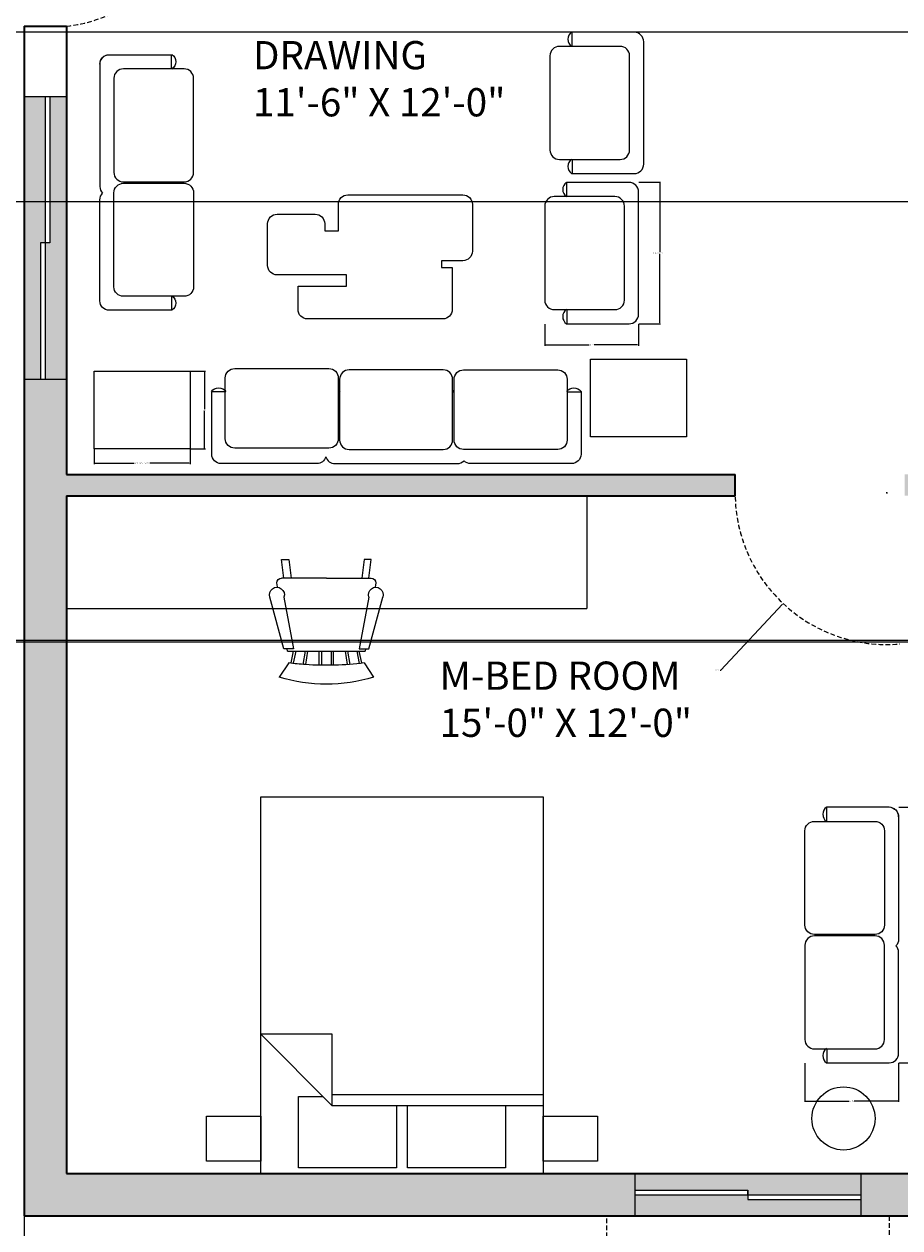
# Model space of a CAD drawing. Units: inches. Extents: x 1693 to 2974, y 2201 to 2965.
# Tile 17 of 24: x 2479 to 2665, y 2332 to 2588. Entities that reach past the tile are written whole.
import ezdxf

# ---------------------------------------------------------------- set-up
doc = ezdxf.new("R2010")
doc.units = ezdxf.units.IN
doc.header["$LTSCALE"] = 2
doc.header["$MEASUREMENT"] = 0
doc.linetypes.add('HIDDEN', pattern=[0.375, 0.25, -0.125])
for name, color, linetype, lineweight in [('A-ANNO-DIMS', 2, 'Continuous', 18), ('A-AREA-IDEN', 7, 'Continuous', 18), ('A-DOOR-SWNG', 3, 'HIDDEN', 13), ('A-FLOR-CASE', 32, 'Continuous', 18), ('A-FURN', 8, 'Continuous', 18), ('A-GLAZ', 4, 'Continuous', 18), ('A-GLAZ-OVHD', 8, 'HIDDEN', 13), ('A-WALL', 7, 'Continuous', 35)]:
    doc.layers.add(name, color=color, linetype=linetype, lineweight=lineweight)
doc.layers.add('A-GLAZ-PATT', color=141, linetype='Continuous', lineweight=13, true_color=0xadddf7)
doc.layers.add('A-WALL-PATT', color=251, linetype='Continuous', lineweight=13, true_color=0x636466)
doc.styles.get("Standard").update_dxf_attribs({"font": 'arial.ttf'})
doc.dimstyles.get("Standard").update_dxf_attribs({"dimtxt": 0.18, "dimasz": 0.18, "dimexe": 0.18, "dimexo": 0.0625, "dimgap": 0.09, "dimtad": 0, "dimtih": 1, "dimtoh": 1, "dimdec": 1, "dimzin": 0, "dimdsep": 46, "dimlunit": 3, "dimtxsty": 'Standard', "dimcen": 0.09, "dimadec": 0, "dimazin": 0, "dimtfac": 1, "dimtdec": 1, "dimtofl": 0, "dimtmove": 0, "dimatfit": 3, "dimfxl": 1, "dimtolj": 1, "dimtzin": 0, "dimarcsym": 0})

# ---------------------------------------------------------------- blocks, each defined once
blk = doc.blocks.new('Chair - Rocking')
for p, q in [((-8, -4.5), (-10, -1.5)), ((8, -4.5), (10, -1.5)), ((-7.5, -4.5), (-7, -7)), ((-6.5, -7), (-7.02225, -4.43)), ((-4.5, -7), (-4.96674, -4.19951)), ((-4, -7), (-4.40532, -4.16272)), ((-1.5, -4.05012), (-1.5, -7)), ((-1, -7), (-1, -4.05012)), ((1, -7), (1, -4.04655)), ((1.5, -4.05012), (1.5, -7)), ((4, -7), (4.40187, -4.18694)), ((4.5, -7), (4.96761, -4.19437)), ((6.5, -7), (7, -4.4057)), ((7.5, -4.5), (7, -7)), ((-9, -7.5), (-12, -18.49999)), ((-7, -7.5), (-9, -7.5)), ((-9, -18.49999), (-7, -7.5)), ((-8.23428, -6.99939), (-8.3093, -7.47958)), ((-8.23041, -7), (8.23915, -7)), ((7, -7.5), (9, -7.5)), ((9, -18.49999), (7, -7.5)), ((8.31071, -7.48854), (8.23449, -7.00073)), ((9, -7.5), (12, -18.49999)), ((-10.36644, -20.64523), (-10.5, -21.49999)), ((-9, -22.49999), (-9.5, -26.49999)), ((0, -22.49999), (-9.5, -22.49999)), ((-8, -26.49999), (-7.5, -22.49999)), ((0, -22.49999), (9.5, -22.49999)), ((8, -26.49999), (7.5, -22.49999)), ((9, -22.49999), (9.5, -26.49999)), ((10.5, -21.49999), (10.3575, -20.58798)), ((-9.5, -26.49999), (-8, -26.49999)), ((9.5, -26.49999), (8, -26.49999))]:
    blk.add_line(p, q)
for centre, radius, start, end in [((0, -34.08333), 34.08333, 72.93847, 107.0615), ((0, -68.25004), 64.25, 93.92211, 97.15267), ((0, -68.25004), 64.25, 82.84733, 93.92211), ((-10.5, -18.99999), 1.58114, 161.5651, 18.43495), ((10.5, -18.99999), 1.58114, 161.5651, 18.43495), ((-9.5, -21.49999), 1, 180, 270), ((9.5, -21.49999), 1, 270, 0)]:
    blk.add_arc(centre, radius, start, end)
blk = doc.blocks.new('Bed - Queen')
for p, q in [((0, -80.00003), (0, 0)), ((0, 0), (59.99999, 0)), ((59.99999, 0), (59.99999, -80.00003)), ((7.99999, -1.2), (28.79998, -1.2)), ((7.99999, -14.4), (7.99999, -1.2)), ((28.79998, -1.2), (28.79998, -14.4)), ((31.19999, -1.2), (51.99999, -1.2)), ((31.19999, -14.4), (31.19999, -1.2)), ((51.99999, -1.2), (51.99999, -16.4)), ((0, -14.4), (44.8, -14.4)), ((59.99999, -29.6), (44.8, -14.4)), ((44.8, -14.4), (44.8, -29.6)), ((44.8, -16.8), (0, -16.8)), ((51.99999, -16.4), (46.79936, -16.4)), ((44.8, -29.6), (59.99999, -29.6)), ((59.99999, -80.00003), (0, -80.00003))]:
    blk.add_line(p, q)
blk = doc.blocks.new('SOFA-2-SEAT')
at = {"ltscale": 2}
for p, q in [((17.9, 54.27), (4.68, 54.27)), ((4.68, 51.27), (4.68, 54.27)), ((4.68, 51.27), (4.68, 51.55)), ((4.68, 27.26), (4.68, 26.96)), ((19.9, 2), (19.9, 23.43)), ((4.68, 3), (4.68, 0)), ((4.59, 0), (17.9, 0))]:
    blk.add_line(p, q, dxfattribs=at)
for points in [[(18.47, 54.18, -0.331344), (19.9, 52.27), (19.9, 26.26, -0.198912), (19.31, 24.85)], [(0, 49.27, -0.414214), (2, 51.27), (14.9, 51.27, -0.414214), (16.9, 49.27), (16.9, 29.26, -0.414214), (14.9, 27.26), (2, 27.26, -0.414214), (0, 29.26), (0, 49.27)], [(0, 4.95, 0.414214), (2, 2.95), (14.9, 2.95, 0.414214), (16.9, 4.95), (16.9, 24.96, 0.414214), (14.9, 26.96), (2, 26.96, 0.414214), (0, 24.96), (0, 4.95)]]:
    blk.add_lwpolyline(points, format="xyb", dxfattribs=at)
for centre, radius, start, end in [((5.65, 52.79), 1.86, 125.0084, 234.9916), ((17.9, 52.27), 2, 0, 90), ((5.65, 52.75), 1.86, 219.881, 234.9916), ((5.65, 25.74), 1.86, 125.0084, 139.1343), ((17.9, 23.43), 2, 0, 45), ((5.65, 1.52), 1.86, 125.0084, 234.9916), ((17.9, 2), 2, 270, 0)]:
    blk.add_arc(centre, radius, start, end, dxfattribs=at)
blk = doc.blocks.new('SOFA-3-SEAT')
at = {"ltscale": 2}
for p, q in [((0.05, 18.19), (0.05, 4.98)), ((22.37, 20.19), (2.05, 20.19)), ((76.47, 20.19), (55.04, 20.19)), ((78.47, 4.88), (78.47, 18.19)), ((3.05, 4.98), (0.05, 4.98)), ((27.21, 4.98), (26.92, 4.98)), ((51.21, 4.98), (51.52, 4.98)), ((75.47, 4.98), (78.47, 4.98))]:
    blk.add_line(p, q, dxfattribs=at)
for points in [[(24.29, 18.76, -0.331344), (26.21, 20.19), (52.21, 20.19, -0.198912), (53.63, 19.6)], [(24.92, 0, 0.414214), (26.92, 2), (26.92, 14.9, 0.414214), (24.92, 16.9), (4.92, 16.9, 0.414214), (2.92, 14.9), (2.92, 2, 0.414214), (4.92, 0), (24.92, 0)], [(29.21, 0.29, -0.414214), (27.21, 2.29), (27.21, 15.19, -0.414214), (29.21, 17.19), (49.21, 17.19, -0.414214), (51.21, 15.19), (51.21, 2.29, -0.414214), (49.21, 0.29), (29.21, 0.29)], [(73.52, 0.29, 0.414214), (75.52, 2.29), (75.52, 15.19, 0.414214), (73.52, 17.19), (53.52, 17.19, 0.414214), (51.52, 15.19), (51.52, 2.29, 0.414214), (53.52, 0.29), (73.52, 0.29)]]:
    blk.add_lwpolyline(points, format="xyb", dxfattribs=at)
for centre, radius, start, end in [((2.05, 18.19), 2, 90, 180), ((22.37, 18.19), 2, 16.6709, 90), ((55.04, 18.19), 2, 90, 135), ((76.47, 18.19), 2, 0, 90), ((1.52, 5.95), 1.86, 215.0084, 324.9916), ((25.73, 5.95), 1.86, 309.881, 324.9916), ((52.73, 5.95), 1.86, 215.0084, 229.1343), ((76.95, 5.95), 1.86, 215.0084, 324.9916)]:
    blk.add_arc(centre, radius, start, end, dxfattribs=at)
blk = doc.blocks.new('LOUNGE-CHAIR-B')
at = {"ltscale": 2}
for p, q in [((4.68, 27.01), (4.68, 30.01)), ((4.68, 3), (4.68, 0))]:
    blk.add_line(p, q, dxfattribs=at)
for points in [[(4.59, 0), (17.9, 0, 0.414214), (19.9, 2), (19.9, 28.01, 0.414214), (17.9, 30.01), (4.68, 30.01)], [(0, 5, 0.414214), (2, 3), (14.9, 3, 0.414214), (16.9, 5), (16.9, 25.01, 0.414214), (14.9, 27.01), (2, 27.01, 0.414214), (0, 25.01), (0, 5)]]:
    blk.add_lwpolyline(points, format="xyb", dxfattribs=at)
for centre in [(5.66, 28.53), (5.66, 1.52)]:
    blk.add_arc(centre, 1.86, 125.0084, 234.9916, dxfattribs=at)
blk = doc.blocks.new('NIGHTSTAND')
at = {"ltscale": 2}
blk.add_lwpolyline([(11.51, 0), (0, 0), (0, 9.62), (11.51, 9.62)], close=True, dxfattribs=at)
blk = doc.blocks.new('TABLE-COCKTAIL')
at = {"ltscale": 2}
blk.add_lwpolyline([(17.32, 26.34), (41.47, 26.34, -0.414214), (43.47, 24.34), (43.47, 14.36, -0.414214), (41.47, 12.36), (36.89, 12.36), (36.89, 10.89), (39.2, 10.89), (39.2, 2, -0.414214), (37.2, 0), (8.45, 0, -0.414214), (6.45, 2), (6.45, 6.97), (16.72, 6.97), (16.72, 9.34), (2, 9.34, -0.414214), (0, 11.34), (0, 20.23, -0.414214), (2, 22.23), (10.11, 22.23, -0.414214), (12.11, 20.23), (12.11, 18.68), (15.01, 18.68), (15.01, 24.34, -0.414214), (17.01, 26.34), (17.32, 26.34)], format="xyb", dxfattribs=at)
blk = doc.blocks.new('TABLE-END-RECT')
at = {"ltscale": 2}
blk.add_lwpolyline([(0, 16.48), (20.41, 16.48), (20.41, 0), (0, 0)], close=True, dxfattribs=at)
blk = doc.blocks.new('TABLE-END-ROUND')
at = {"ltscale": 2}
blk.add_circle((6.71, 6.71), 6.71, dxfattribs=at)
blk = doc.blocks.new('*D47')
at = {"layer": 'A-ANNO-DIMS', "color": 0, "lineweight": -2, "ltscale": 2, "transparency": 16777216}
for p, q in [((2665.02, 2421.61), (2673.28, 2421.61)), ((2673.1, 2421.43), (2673.1, 2394.63)), ((2673.1, 2367.47), (2673.1, 2394.27)), ((2665.02, 2367.29), (2673.28, 2367.29))]:
    blk.add_line(p, q, dxfattribs=at)
at = {"layer": 'A-ANNO-DIMS', "color": 0, "ltscale": 2, "transparency": 16777216}
for points in [[(2673.07, 2421.43), (2673.13, 2421.43), (2673.1, 2421.61)], [(2673.07, 2367.47), (2673.13, 2367.47), (2673.1, 2367.29)]]:
    blk.add_solid(points, dxfattribs=at)
at = {"layer": 'Defpoints', "color": 0, "ltscale": 2, "transparency": 16777216}
for p in [(2664.96, 2421.61), (2673.1, 2421.61), (2664.96, 2367.29)]:
    blk.add_point(p, dxfattribs=at)
at = {"layer": 'A-ANNO-DIMS', "color": 0, "ltscale": 2, "transparency": 16777216, "insert": (2673.1, 2394.45), "char_height": 0.18, "attachment_point": 5}
blk.add_mtext('\\A1;TWO-SEAT SOFA 54 TYP.', dxfattribs=at)
blk = doc.blocks.new('*D48')
at = {"layer": 'A-ANNO-DIMS', "color": 0, "lineweight": -2, "ltscale": 2, "transparency": 16777216}
for p, q in [((2645.06, 2367.23), (2645.06, 2358.97)), ((2664.96, 2367.23), (2664.96, 2358.97)), ((2645.24, 2359.15), (2654.48, 2359.15)), ((2664.78, 2359.15), (2655.54, 2359.15))]:
    blk.add_line(p, q, dxfattribs=at)
at = {"layer": 'A-ANNO-DIMS', "color": 0, "ltscale": 2, "transparency": 16777216}
for points in [[(2645.24, 2359.18), (2645.24, 2359.12), (2645.06, 2359.15)], [(2664.78, 2359.18), (2664.78, 2359.12), (2664.96, 2359.15)]]:
    blk.add_solid(points, dxfattribs=at)
at = {"layer": 'Defpoints', "color": 0, "ltscale": 2, "transparency": 16777216}
for p in [(2645.06, 2367.29), (2664.96, 2367.29), (2664.96, 2359.15)]:
    blk.add_point(p, dxfattribs=at)
at = {"layer": 'A-ANNO-DIMS', "color": 0, "ltscale": 2, "transparency": 16777216, "insert": (2655.01, 2359.15), "char_height": 0.18, "attachment_point": 5}
blk.add_mtext('\\A1;20 TYP.', dxfattribs=at)
blk = doc.blocks.new('*D67')
at = {"layer": 'A-ANNO-DIMS', "color": 0, "lineweight": -2, "ltscale": 2, "transparency": 16777216}
for p, q in [((2609.78, 2554.32), (2614.41, 2554.32)), ((2614.23, 2554.14), (2614.23, 2539.48)), ((2614.23, 2524.45), (2614.23, 2539.11)), ((2609.78, 2524.27), (2614.41, 2524.27))]:
    blk.add_line(p, q, dxfattribs=at)
at = {"layer": 'A-ANNO-DIMS', "color": 0, "ltscale": 2, "transparency": 16777216}
for points in [[(2614.2, 2554.14), (2614.26, 2554.14), (2614.23, 2554.32)], [(2614.2, 2524.45), (2614.26, 2524.45), (2614.23, 2524.27)]]:
    blk.add_solid(points, dxfattribs=at)
at = {"layer": 'Defpoints', "color": 0, "ltscale": 2, "transparency": 16777216}
for p in [(2609.72, 2554.32), (2614.23, 2554.32), (2609.72, 2524.27)]:
    blk.add_point(p, dxfattribs=at)
at = {"layer": 'A-ANNO-DIMS', "color": 0, "ltscale": 2, "transparency": 16777216, "insert": (2614.23, 2539.3), "char_height": 0.18, "attachment_point": 5}
blk.add_mtext('\\A1;LOUNGE CHAIR B 30 TYP.', dxfattribs=at)
blk = doc.blocks.new('*D68')
at = {"layer": 'A-ANNO-DIMS', "color": 0, "lineweight": -2, "ltscale": 2, "transparency": 16777216}
for p, q in [((2589.82, 2524.21), (2589.82, 2519.58)), ((2609.72, 2524.21), (2609.72, 2519.58)), ((2590, 2519.76), (2599.24, 2519.76)), ((2609.54, 2519.76), (2600.3, 2519.76))]:
    blk.add_line(p, q, dxfattribs=at)
at = {"layer": 'A-ANNO-DIMS', "color": 0, "ltscale": 2, "transparency": 16777216}
for points in [[(2590, 2519.79), (2590, 2519.73), (2589.82, 2519.76)], [(2609.54, 2519.79), (2609.54, 2519.73), (2609.72, 2519.76)]]:
    blk.add_solid(points, dxfattribs=at)
at = {"layer": 'Defpoints', "color": 0, "ltscale": 2, "transparency": 16777216}
for p in [(2589.82, 2524.27), (2609.72, 2524.27), (2609.72, 2519.76)]:
    blk.add_point(p, dxfattribs=at)
at = {"layer": 'A-ANNO-DIMS', "color": 0, "ltscale": 2, "transparency": 16777216, "insert": (2599.77, 2519.76), "char_height": 0.18, "attachment_point": 5}
blk.add_mtext('\\A1;20 TYP.', dxfattribs=at)
blk = doc.blocks.new('*D73')
at = {"layer": 'A-ANNO-DIMS', "color": 0, "lineweight": -2, "ltscale": 2, "transparency": 16777216}
for p, q in [((2494.1, 2497.64), (2494.1, 2494.46)), ((2514.51, 2497.64), (2514.51, 2494.46)), ((2494.28, 2494.64), (2502.64, 2494.64)), ((2514.33, 2494.64), (2505.97, 2494.64))]:
    blk.add_line(p, q, dxfattribs=at)
at = {"layer": 'A-ANNO-DIMS', "color": 0, "ltscale": 2, "transparency": 16777216}
for points in [[(2494.28, 2494.67), (2494.28, 2494.61), (2494.1, 2494.64)], [(2514.33, 2494.67), (2514.33, 2494.61), (2514.51, 2494.64)]]:
    blk.add_solid(points, dxfattribs=at)
at = {"layer": 'Defpoints', "color": 0, "ltscale": 2, "transparency": 16777216}
for p in [(2494.1, 2497.7), (2514.51, 2497.7), (2514.51, 2494.64)]:
    blk.add_point(p, dxfattribs=at)
at = {"layer": 'A-ANNO-DIMS', "color": 0, "ltscale": 2, "transparency": 16777216, "insert": (2504.31, 2494.64), "char_height": 0.18, "attachment_point": 5}
blk.add_mtext('\\A1;RECT. END TABLE 20 TYP.', dxfattribs=at)
blk = doc.blocks.new('*D74')
at = {"layer": 'A-ANNO-DIMS', "color": 0, "lineweight": -2, "ltscale": 2, "transparency": 16777216}
for p, q in [((2514.57, 2514.18), (2517.75, 2514.18)), ((2517.57, 2514), (2517.57, 2506.12)), ((2517.57, 2497.88), (2517.57, 2505.76)), ((2514.57, 2497.7), (2517.75, 2497.7))]:
    blk.add_line(p, q, dxfattribs=at)
at = {"layer": 'A-ANNO-DIMS', "color": 0, "ltscale": 2, "transparency": 16777216}
for points in [[(2517.54, 2514), (2517.6, 2514), (2517.57, 2514.18)], [(2517.54, 2497.88), (2517.6, 2497.88), (2517.57, 2497.7)]]:
    blk.add_solid(points, dxfattribs=at)
at = {"layer": 'Defpoints', "color": 0, "ltscale": 2, "transparency": 16777216}
for p in [(2514.51, 2514.18), (2517.57, 2514.18), (2514.51, 2497.7)]:
    blk.add_point(p, dxfattribs=at)
at = {"layer": 'A-ANNO-DIMS', "color": 0, "ltscale": 2, "transparency": 16777216, "insert": (2517.57, 2505.94), "char_height": 0.18, "attachment_point": 5}
blk.add_mtext('\\A1;16 TYP.', dxfattribs=at)
blk = doc.blocks.new('*D81')
at = {"layer": 'A-ANNO-DIMS', "color": 0, "lineweight": -2, "ltscale": 2, "transparency": 16777216}
for p, q in [((1752.34, 2553.91), (1752.34, 2964.96)), ((1752.52, 2964.78), (2332.94, 2964.78)), ((2914.06, 2964.78), (2333.64, 2964.78)), ((2914.24, 2754.97), (2914.24, 2964.96))]:
    blk.add_line(p, q, dxfattribs=at)
at = {"layer": 'A-ANNO-DIMS', "color": 0, "ltscale": 2, "transparency": 16777216}
for points in [[(1752.52, 2964.81), (1752.52, 2964.75), (1752.34, 2964.78)], [(2914.06, 2964.81), (2914.06, 2964.75), (2914.24, 2964.78)]]:
    blk.add_solid(points, dxfattribs=at)
at = {"layer": 'Defpoints', "color": 0, "ltscale": 2, "transparency": 16777216}
for p in [(2914.24, 2964.78), (2914.24, 2754.9), (1752.34, 2553.84)]:
    blk.add_point(p, dxfattribs=at)
at = {"layer": 'A-ANNO-DIMS', "color": 0, "ltscale": 2, "transparency": 16777216, "insert": (2333.29, 2964.78), "char_height": 0.18, "attachment_point": 5}
blk.add_mtext('\\A1;1162', dxfattribs=at)
blk = doc.blocks.new('*D82')
at = {"layer": 'A-ANNO-DIMS', "color": 0, "lineweight": -2, "ltscale": 2, "transparency": 16777216}
for p, q in [((2615.67, 2906.08), (1693.46, 2906.08)), ((1693.64, 2905.9), (1693.64, 2582.94)), ((1693.64, 2259.62), (1693.64, 2582.58)), ((2096.17, 2259.44), (1693.46, 2259.44))]:
    blk.add_line(p, q, dxfattribs=at)
at = {"layer": 'A-ANNO-DIMS', "color": 0, "ltscale": 2, "transparency": 16777216}
for points in [[(1693.61, 2905.9), (1693.67, 2905.9), (1693.64, 2906.08)], [(1693.61, 2259.62), (1693.67, 2259.62), (1693.64, 2259.44)]]:
    blk.add_solid(points, dxfattribs=at)
at = {"layer": 'Defpoints', "color": 0, "ltscale": 2, "transparency": 16777216}
for p in [(1693.64, 2906.08), (2615.74, 2906.08), (2096.24, 2259.44)]:
    blk.add_point(p, dxfattribs=at)
at = {"layer": 'A-ANNO-DIMS', "color": 0, "ltscale": 2, "transparency": 16777216, "insert": (1693.64, 2582.76), "char_height": 0.18, "attachment_point": 5}
blk.add_mtext('\\A1;646.6', dxfattribs=at)
blk = doc.blocks.new('*D85')
at = {"layer": 'A-ANNO-DIMS', "color": 0, "lineweight": -2, "ltscale": 2, "transparency": 16777216}
for p, q in [((2479.24, 2334.69), (2479.24, 2200.56)), ((2902.24, 2334.69), (2902.24, 2200.56)), ((2479.42, 2200.74), (2690.44, 2200.74)), ((2902.06, 2200.74), (2691.03, 2200.74))]:
    blk.add_line(p, q, dxfattribs=at)
at = {"layer": 'A-ANNO-DIMS', "color": 0, "ltscale": 2, "transparency": 16777216}
for points in [[(2479.42, 2200.77), (2479.42, 2200.71), (2479.24, 2200.74)], [(2902.06, 2200.77), (2902.06, 2200.71), (2902.24, 2200.74)]]:
    blk.add_solid(points, dxfattribs=at)
at = {"layer": 'Defpoints', "color": 0, "ltscale": 2, "transparency": 16777216}
for p in [(2479.24, 2334.75), (2902.24, 2334.75), (2902.24, 2200.74)]:
    blk.add_point(p, dxfattribs=at)
at = {"layer": 'A-ANNO-DIMS', "color": 0, "ltscale": 2, "transparency": 16777216, "insert": (2690.74, 2200.74), "char_height": 0.18, "attachment_point": 5}
blk.add_mtext('\\A1;423', dxfattribs=at)
blk = doc.blocks.new('*D89')
at = {"layer": 'A-ANNO-DIMS', "color": 0, "lineweight": -2, "ltscale": 2, "transparency": 16777216}
for p, q in [((2479.3, 2334.75), (2973.12, 2334.75)), ((2972.94, 2334.57), (2972.94, 2312.48)), ((2972.94, 2290.02), (2972.94, 2312.12)), ((2294.3, 2289.84), (2973.12, 2289.84))]:
    blk.add_line(p, q, dxfattribs=at)
at = {"layer": 'A-ANNO-DIMS', "color": 0, "ltscale": 2, "transparency": 16777216}
for points in [[(2972.91, 2334.57), (2972.97, 2334.57), (2972.94, 2334.75)], [(2972.91, 2290.02), (2972.97, 2290.02), (2972.94, 2289.84)]]:
    blk.add_solid(points, dxfattribs=at)
at = {"layer": 'Defpoints', "color": 0, "ltscale": 2, "transparency": 16777216}
for p in [(2479.24, 2334.75), (2972.94, 2334.75), (2294.24, 2289.84)]:
    blk.add_point(p, dxfattribs=at)
at = {"layer": 'A-ANNO-DIMS', "color": 0, "ltscale": 2, "transparency": 16777216, "insert": (2972.94, 2312.3), "char_height": 0.18, "attachment_point": 5}
blk.add_mtext('\\A1;44.91', dxfattribs=at)
blk = doc.blocks.new('*D96')
at = {"layer": 'A-ANNO-DIMS', "color": 0, "lineweight": -2, "ltscale": 2, "transparency": 16777216}
for p, q in [((2294.3, 2586.26), (2973.12, 2586.26)), ((2972.94, 2586.08), (2972.94, 2568.45)), ((2972.94, 2550.44), (2972.94, 2568.08)), ((2294.3, 2550.26), (2973.12, 2550.26))]:
    blk.add_line(p, q, dxfattribs=at)
at = {"layer": 'A-ANNO-DIMS', "color": 0, "ltscale": 2, "transparency": 16777216}
for points in [[(2972.91, 2586.08), (2972.97, 2586.08), (2972.94, 2586.26)], [(2972.91, 2550.44), (2972.97, 2550.44), (2972.94, 2550.26)]]:
    blk.add_solid(points, dxfattribs=at)
at = {"layer": 'Defpoints', "color": 0, "ltscale": 2, "transparency": 16777216}
for p in [(2294.24, 2586.26), (2972.94, 2586.26), (2294.24, 2550.26)]:
    blk.add_point(p, dxfattribs=at)
at = {"layer": 'A-ANNO-DIMS', "color": 0, "ltscale": 2, "transparency": 16777216, "insert": (2972.94, 2568.26), "char_height": 0.18, "attachment_point": 5}
blk.add_mtext('\\A1;36', dxfattribs=at)
blk = doc.blocks.new('*D97')
at = {"layer": 'A-ANNO-DIMS', "color": 0, "lineweight": -2, "ltscale": 2, "transparency": 16777216}
for p, q in [((2294.3, 2631.75), (2973.12, 2631.75)), ((2972.94, 2631.57), (2972.94, 2609.19)), ((2972.94, 2586.44), (2972.94, 2608.83)), ((2294.3, 2586.26), (2973.12, 2586.26))]:
    blk.add_line(p, q, dxfattribs=at)
at = {"layer": 'A-ANNO-DIMS', "color": 0, "ltscale": 2, "transparency": 16777216}
for points in [[(2972.91, 2631.57), (2972.97, 2631.57), (2972.94, 2631.75)], [(2972.91, 2586.44), (2972.97, 2586.44), (2972.94, 2586.26)]]:
    blk.add_solid(points, dxfattribs=at)
at = {"layer": 'Defpoints', "color": 0, "ltscale": 2, "transparency": 16777216}
for p in [(2294.24, 2631.75), (2972.94, 2631.75), (2294.24, 2586.26)]:
    blk.add_point(p, dxfattribs=at)
at = {"layer": 'A-ANNO-DIMS', "color": 0, "ltscale": 2, "transparency": 16777216, "insert": (2972.94, 2609.01), "char_height": 0.18, "attachment_point": 5}
blk.add_mtext('\\A1;45.49', dxfattribs=at)
blk = doc.blocks.new('*D108')
at = {"layer": 'A-ANNO-DIMS', "color": 0, "lineweight": -2, "ltscale": 2, "transparency": 16777216}
for p, q in [((2972.94, 2457.27), (2972.94, 2457.45)), ((2972.94, 2457.45), (2973.12, 2457.45)), ((1752.74, 2457.09), (2973.12, 2457.09)), ((1752.74, 2456.73), (2973.12, 2456.73)), ((2972.94, 2456.55), (2972.94, 2456.37))]:
    blk.add_line(p, q, dxfattribs=at)
at = {"layer": 'A-ANNO-DIMS', "color": 0, "ltscale": 2, "transparency": 16777216}
for points in [[(2972.91, 2457.27), (2972.97, 2457.27), (2972.94, 2457.09)], [(2972.91, 2456.55), (2972.97, 2456.55), (2972.94, 2456.73)]]:
    blk.add_solid(points, dxfattribs=at)
at = {"layer": 'Defpoints', "color": 0, "ltscale": 2, "transparency": 16777216}
for p in [(1752.68, 2457.09), (1752.68, 2456.73), (2972.94, 2457.09)]:
    blk.add_point(p, dxfattribs=at)
at = {"layer": 'A-ANNO-DIMS', "color": 0, "ltscale": 2, "transparency": 16777216, "insert": (2973.44, 2457.45), "char_height": 0.18, "attachment_point": 5}
blk.add_mtext('\\A1;0.36', dxfattribs=at)
blk = doc.blocks.new('*D115')
at = {"layer": 'A-ANNO-DIMS', "color": 0, "lineweight": -2, "ltscale": 2, "transparency": 16777216}
for p, q in [((2662.4, 2488.39), (2662.58, 2488.39)), ((2662.49, 2488.3), (2662.49, 2488.48)), ((2627.21, 2450.72), (2640.31, 2464.72)), ((2627.03, 2450.72), (2627.21, 2450.72))]:
    blk.add_line(p, q, dxfattribs=at)
at = {"layer": 'A-ANNO-DIMS', "color": 0, "ltscale": 2, "transparency": 16777216}
blk.add_solid([(2640.29, 2464.74), (2640.34, 2464.7), (2640.44, 2464.85)], dxfattribs=at)
at = {"layer": 'Defpoints', "color": 0, "ltscale": 2, "transparency": 16777216}
for p in [(2662.49, 2488.39), (2640.44, 2464.85)]:
    blk.add_point(p, dxfattribs=at)
at = {"layer": 'A-ANNO-DIMS', "color": 0, "ltscale": 2, "transparency": 16777216, "insert": (2626.48, 2450.72), "char_height": 0.18, "attachment_point": 5}
blk.add_mtext('\\A1;R32.256', dxfattribs=at)

msp = doc.modelspace()

# ---------------------------------------------------------------- hatches: boundary and pattern name
at = {"layer": 'A-GLAZ-PATT', "ltscale": 2}
h = msp.add_hatch(color=256, dxfattribs=at)
h.dxf.hatch_style = 1
h.paths.add_polyline_path([(2656.9702, 2338.2547), (2632.9702, 2338.2547), (2632.9702, 2339.2547), (2608.9702, 2339.2547), (2608.9702, 2334.7547), (2656.9702, 2334.7547)])
h.paths.add_polyline_path([(2656.9702, 2343.7547), (2608.9702, 2343.7547), (2608.9702, 2340.2547), (2632.9702, 2340.2547), (2632.9702, 2339.2547), (2656.9702, 2339.2547)])
h.paths.add_polyline_path([(2775.7544, 2338.2547), (2751.7544, 2338.2547), (2751.7544, 2334.7547), (2775.7544, 2334.7547)])
h.paths.add_polyline_path([(2775.7544, 2343.7547), (2751.7544, 2343.7547), (2751.7544, 2340.2547), (2775.7544, 2340.2547)])
h.paths.add_polyline_path([(2897.7363, 2568.7999), (2893.2363, 2568.7999), (2893.2363, 2520.7999), (2896.7363, 2520.7999), (2896.7363, 2544.7999), (2897.7363, 2544.7999)])
h.paths.add_polyline_path([(2902.2363, 2568.7999), (2898.7363, 2568.7999), (2898.7363, 2544.7999), (2897.7363, 2544.7999), (2897.7363, 2520.7999), (2902.2363, 2520.7999)])
h.paths.add_polyline_path([(2902.2363, 2637.7547), (2898.7363, 2637.7547), (2898.7363, 2613.7547), (2902.2363, 2613.7547)])
h.paths.add_polyline_path([(2896.7363, 2637.7547), (2893.2363, 2637.7547), (2893.2363, 2613.7547), (2896.7363, 2613.7547)])
h.paths.add_polyline_path([(2902.2363, 2748.903), (2899.0477, 2748.903), (2899.0477, 2724.903), (2898.0477, 2724.903), (2898.0477, 2700.903), (2902.2363, 2700.903)])
h.paths.add_polyline_path([(2898.0477, 2748.903), (2893.2363, 2748.903), (2893.2363, 2700.903), (2897.0477, 2700.903), (2897.0477, 2724.903), (2898.0477, 2724.903)])
h.paths.add_polyline_path([(2851.2363, 2846.2547), (2803.2363, 2846.2547), (2803.2363, 2842.7547), (2827.2363, 2842.7547), (2827.2363, 2841.7547), (2851.2363, 2841.7547)])
h.paths.add_polyline_path([(2851.2363, 2840.7547), (2827.2363, 2840.7547), (2827.2363, 2841.7547), (2803.2363, 2841.7547), (2803.2363, 2837.2547), (2851.2363, 2837.2547)])
h.paths.add_polyline_path([(2578.2363, 2846.2547), (2530.2363, 2846.2547), (2530.2363, 2842.7547), (2554.2363, 2842.7547), (2554.2363, 2841.7547), (2578.2363, 2841.7547)])
h.paths.add_polyline_path([(2578.2363, 2840.7547), (2554.2363, 2840.7547), (2554.2363, 2841.7547), (2530.2363, 2841.7547), (2530.2363, 2837.2547), (2578.2363, 2837.2547)])
h.paths.add_polyline_path([(2732.7363, 2812.7547), (2705.1363, 2812.7547), (2705.1363, 2811.7547), (2676.3363, 2811.7547), (2676.3363, 2812.7547), (2648.7363, 2812.7547), (2648.7363, 2808.2547), (2732.7363, 2808.2547)])
h.paths.add_polyline_path([(2732.7363, 2817.2547), (2648.7363, 2817.2547), (2648.7363, 2813.7547), (2676.3363, 2813.7547), (2676.3363, 2812.7547), (2705.1363, 2812.7547), (2705.1363, 2813.7547), (2732.7363, 2813.7547)])
h.paths.add_polyline_path([(2488.2363, 2695.8203), (2484.7878, 2695.8203), (2484.7878, 2671.8203), (2488.2363, 2671.8203)])
h.paths.add_polyline_path([(2482.7878, 2695.8203), (2479.2363, 2695.8203), (2479.2363, 2671.8203), (2482.7878, 2671.8203)])
h.paths.add_polyline_path([(2488.2363, 2572.4371), (2484.7363, 2572.4371), (2484.7363, 2541.4371), (2483.7363, 2541.4371), (2483.7363, 2512.4371), (2488.2363, 2512.4371)])
h.paths.add_polyline_path([(2482.7363, 2541.4371), (2483.7363, 2541.4371), (2483.7363, 2572.4371), (2479.2363, 2572.4371), (2479.2363, 2512.4371), (2482.7363, 2512.4371)])
h.paths.add_polyline_path([(2248.9863, 2706.8449), (2190.9863, 2706.8449), (2190.9863, 2703.3449), (2219.9863, 2703.3449), (2219.9863, 2702.3449), (2248.9863, 2702.3449)])
h.paths.add_polyline_path([(2248.9863, 2701.3449), (2219.9863, 2701.3449), (2219.9863, 2702.3449), (2190.9863, 2702.3449), (2190.9863, 2697.8449), (2248.9863, 2697.8449)])
h.paths.add_polyline_path([(2151.9207, 2293.3449), (2127.9207, 2293.3449), (2127.9207, 2289.8449), (2151.9207, 2289.8449)])
h.paths.add_polyline_path([(2151.9207, 2298.8449), (2127.9207, 2298.8449), (2127.9207, 2295.3449), (2151.9207, 2295.3449)])
h.paths.add_polyline_path([(2084.023, 2293.3449), (2066.023, 2293.3449), (2066.023, 2294.3449), (2048.023, 2294.3449), (2048.023, 2289.8449), (2084.023, 2289.8449)])
h.paths.add_polyline_path([(2084.023, 2298.8449), (2048.023, 2298.8449), (2048.023, 2295.3449), (2066.023, 2295.3449), (2066.023, 2294.3449), (2084.023, 2294.3449)])
h.paths.add_polyline_path([(1966.0781, 2293.3449), (1948.0781, 2293.3449), (1948.0781, 2294.3449), (1930.0781, 2294.3449), (1930.0781, 2289.8449), (1966.0781, 2289.8449)])
h.paths.add_polyline_path([(1966.0781, 2298.8449), (1930.0781, 2298.8449), (1930.0781, 2295.3449), (1948.0781, 2295.3449), (1948.0781, 2294.3449), (1966.0781, 2294.3449)])
h.paths.add_polyline_path([(1787.2363, 2403.1922), (1782.7363, 2403.1922), (1782.7363, 2355.1922), (1786.2363, 2355.1922), (1786.2363, 2379.1922), (1787.2363, 2379.1922)])
h.paths.add_polyline_path([(1791.7363, 2403.1922), (1788.2363, 2403.1922), (1788.2363, 2379.1922), (1787.2363, 2379.1922), (1787.2363, 2355.1922), (1791.7363, 2355.1922)])
h.paths.add_polyline_path([(1786.2363, 2477.5455), (1782.7363, 2477.5455), (1782.7363, 2453.5455), (1786.2363, 2453.5455)])
h.paths.add_polyline_path([(1791.7363, 2477.5455), (1788.2363, 2477.5455), (1788.2363, 2453.5455), (1791.7363, 2453.5455)])
h.paths.add_polyline_path([(1786.2363, 2621.6433), (1782.7363, 2621.6433), (1782.7363, 2585.6433), (1786.2363, 2585.6433)])
h.paths.add_polyline_path([(1791.7363, 2621.6433), (1788.2363, 2621.6433), (1788.2363, 2585.6433), (1791.7363, 2585.6433)])
h.paths.add_polyline_path([(1908.1286, 2706.8449), (1860.1286, 2706.8449), (1860.1286, 2703.3449), (1884.1286, 2703.3449), (1884.1286, 2702.3449), (1908.1286, 2702.3449)])
h.paths.add_polyline_path([(1908.1286, 2701.3449), (1884.1286, 2701.3449), (1884.1286, 2702.3449), (1860.1286, 2702.3449), (1860.1286, 2697.8449), (1908.1286, 2697.8449)])
h.paths.add_polyline_path([(1973.9863, 2706.8449), (1949.9863, 2706.8449), (1949.9863, 2703.3449), (1973.9863, 2703.3449)])
h.paths.add_polyline_path([(1973.9863, 2701.3449), (1949.9863, 2701.3449), (1949.9863, 2697.8449), (1973.9863, 2697.8449)])
h.paths.add_polyline_path([(2112.7363, 2690.3449), (2028.7363, 2690.3449), (2028.7363, 2686.8449), (2056.3363, 2686.8449), (2056.3363, 2685.8449), (2085.1363, 2685.8449), (2085.1363, 2686.8449), (2112.7363, 2686.8449)])
h.paths.add_polyline_path([(2112.7363, 2685.8449), (2085.1363, 2685.8449), (2085.1363, 2684.8449), (2056.3363, 2684.8449), (2056.3363, 2685.8449), (2028.7363, 2685.8449), (2028.7363, 2681.3449), (2112.7363, 2681.3449)])
h.paths.add_polyline_path([(2422.7363, 2640.7547), (2350.7363, 2640.7547), (2350.7363, 2637.2547), (2386.7363, 2637.2547), (2386.7363, 2636.2547), (2422.7363, 2636.2547)])
h.paths.add_polyline_path([(2422.7363, 2635.2547), (2386.7363, 2635.2547), (2386.7363, 2636.2547), (2350.7363, 2636.2547), (2350.7363, 2631.7547), (2422.7363, 2631.7547)])
at = {"layer": 'A-WALL-PATT', "ltscale": 2}
h = msp.add_hatch(color=256, dxfattribs=at)
h.dxf.hatch_style = 1
h.paths.add_polyline_path([(1928.2363, 2733.2161), (1930.9384, 2733.2161), (1930.9384, 2737.2161), (1923.7363, 2737.2161), (1923.7363, 2706.8449), (1908.1286, 2706.8449), (1908.1286, 2697.8449), (1923.7363, 2697.8449), (1923.7363, 2692.8449), (1928.2363, 2692.8449), (1928.2363, 2697.8449), (1949.9863, 2697.8449), (1949.9863, 2706.8449), (1928.2363, 2706.8449)])
h.paths.add_polyline_path([(2004.7363, 2737.2161), (1995.7363, 2737.2161), (1995.7363, 2706.8449), (1985.6374, 2706.8449), (1973.9863, 2706.8449), (1973.9863, 2697.8449), (2000.2363, 2697.8449), (2000.2363, 2686.5348), (2000.3613, 2686.5348), (2000.3613, 2667.0432), (2000.2363, 2601.8449), (1928.2363, 2601.8449), (1928.2363, 2662.8449), (1923.7363, 2662.8449), (1923.7363, 2595.3449), (1928.2363, 2595.3449), (1928.2363, 2597.3449), (2004.7363, 2597.3449), (2004.7363, 2681.3449), (2012.7814, 2681.3449), (2028.7363, 2681.3449), (2028.7363, 2690.3449), (2004.7363, 2690.3449)])
h.paths.add_polyline_path([(2190.9863, 2706.8449), (2184.9863, 2706.8449), (2145.7363, 2706.8449), (2145.7363, 2765.3449), (2145.7363, 2774.5394), (2136.7363, 2774.5394), (2136.7363, 2756.3449), (2136.7363, 2690.3449), (2112.7363, 2690.3449), (2112.7363, 2681.3449), (2136.7363, 2681.3449), (2136.7363, 2597.3449), (2141.2363, 2597.3449), (2141.2363, 2697.8449), (2190.9863, 2697.8449)])
h.paths.add_polyline_path([(1860.1286, 2706.8449), (1782.7363, 2706.8449), (1782.7363, 2621.6433), (1791.7363, 2621.6433), (1791.7363, 2697.8449), (1860.1286, 2697.8449)])
h.paths.add_polyline_path([(1791.7363, 2585.6433), (1782.7363, 2585.6433), (1782.7363, 2562.8449), (1782.7363, 2553.8449), (1752.3363, 2553.8449), (1752.3363, 2544.2586), (1756.3363, 2544.2586), (1756.3363, 2549.3449), (1782.7363, 2549.3449), (1782.7363, 2489.2404), (1782.7363, 2477.5455), (1791.7363, 2477.5455), (1791.7363, 2493.5991), (1791.6113, 2493.5991), (1791.6113, 2513.0907), (1791.6824, 2533.7198, -0.94742783), (1791.7363, 2534.7168), (1791.7363, 2549.3449), (1863.7363, 2549.3449), (1863.7363, 2513.3449), (1866.7363, 2513.3449), (1866.7363, 2549.3449), (1924.7363, 2549.3449), (1924.7363, 2447.3449), (1924.7363, 2442.8449), (1933.7363, 2442.8449), (1933.7363, 2447.3449), (1928.2363, 2447.3449), (1928.2363, 2559.3449), (1923.7363, 2559.3449), (1923.7363, 2553.8449), (1791.7363, 2553.8449), (1791.7363, 2562.8449)])
h.paths.add_polyline_path([(1791.7363, 2442.8449), (1866.7363, 2442.8449), (1866.7363, 2447.3449), (1866.7363, 2483.3449), (1863.7363, 2483.3449), (1863.7363, 2447.3449), (1791.7363, 2447.3449), (1791.7363, 2453.5455), (1782.7363, 2453.5455), (1782.7363, 2447.3449), (1756.3363, 2447.3449), (1756.3363, 2455.7126), (1752.3363, 2455.7126), (1752.3363, 2442.8449), (1782.7363, 2442.8449), (1782.7363, 2403.1922), (1791.7363, 2403.1922)])
h.paths.add_polyline_path([(1930.0781, 2298.8449), (1791.7363, 2298.8449), (1791.7363, 2355.1922), (1782.7363, 2355.1922), (1782.7363, 2289.8449), (1930.0781, 2289.8449)])
h.paths.add_polyline_path([(2624.7363, 2883.2547), (2624.7363, 2902.6165), (2624.7363, 2906.0761), (2615.7363, 2906.0761), (2615.7363, 2892.2547), (2615.7363, 2846.2547), (2578.2363, 2846.2547), (2578.2363, 2837.2547), (2620.2363, 2837.2547), (2620.2363, 2743.2547), (2624.7363, 2743.2547), (2624.7363, 2808.2547), (2648.7363, 2808.2547), (2648.7363, 2817.2547), (2624.7363, 2817.2547)])
h.paths.add_polyline_path([(2530.2363, 2846.2547), (2479.2363, 2846.2547), (2479.2363, 2695.8203), (2488.2363, 2695.8203), (2488.2363, 2700.7547), (2567.2363, 2700.7547), (2567.2363, 2705.2547), (2488.2363, 2705.2547), (2488.2363, 2837.2547), (2530.2363, 2837.2547)])
h.paths.add_polyline_path([(2488.2363, 2487.7547), (2630.2363, 2487.7547, -0.00990191), (2630.2363, 2489.0322), (2630.2363, 2492.2547), (2488.2363, 2492.2547), (2488.2363, 2512.4371), (2479.2363, 2512.4371), (2479.2363, 2334.7547), (2608.9702, 2334.7547), (2608.9702, 2343.7547), (2488.2363, 2343.7547)])
h.paths.add_polyline_path([(2751.7544, 2343.7547), (2672.7363, 2343.7547), (2672.7363, 2409.7547), (2674.7363, 2409.7547), (2674.7363, 2413.7547), (2672.7363, 2413.7547), (2672.7363, 2487.7547), (2732.7363, 2487.7547), (2732.7363, 2413.7547), (2704.7363, 2413.7547), (2704.7363, 2409.7547), (2784.7363, 2409.7547), (2784.7363, 2343.7547), (2775.7544, 2343.7547), (2775.7544, 2334.7547), (2902.2363, 2334.7547), (2902.2363, 2520.7999), (2893.2363, 2520.7999), (2893.2363, 2413.7547), (2856.0145, 2413.7547), (2856.0145, 2409.7547), (2893.2363, 2409.7547), (2893.2363, 2343.7547), (2789.2363, 2343.7547), (2789.2363, 2409.7547), (2819.2363, 2409.7547), (2826.0145, 2409.7547), (2826.0145, 2413.7547), (2789.2363, 2413.7547), (2789.2363, 2492.2547), (2784.7363, 2492.2547), (2784.7363, 2413.7547), (2736.7363, 2413.7547), (2736.7363, 2492.2547), (2672.7363, 2492.2547), (2666.2363, 2492.2547), (2666.2363, 2487.7547), (2668.2363, 2487.7547), (2668.2363, 2343.7547), (2656.9702, 2343.7547), (2656.9702, 2334.7547), (2662.9702, 2334.7547), (2751.7544, 2334.7547)])
h.paths.add_polyline_path([(2902.2363, 2613.7547), (2893.2363, 2613.7547), (2893.2363, 2589.7547), (2785.2363, 2589.7547), (2785.2363, 2661.7547), (2790.2363, 2661.7547), (2790.2363, 2665.2547), (2761.2363, 2665.2547), (2761.2363, 2667.2547), (2756.7363, 2667.2547), (2756.7363, 2661.7547), (2781.2363, 2661.7547), (2781.2363, 2585.7547), (2893.2363, 2585.7547), (2893.2363, 2568.7999), (2902.2363, 2568.7999)])
h.paths.add_polyline_path([(2488.2363, 2671.8203), (2479.2363, 2671.8203), (2479.2363, 2645.2547), (2479.2363, 2623.4598), (2488.2363, 2623.4598), (2488.2363, 2636.2547), (2624.7363, 2636.2547), (2624.7363, 2640.7547), (2603.7363, 2640.7547), (2603.7363, 2700.7547), (2624.7363, 2700.7547), (2624.7363, 2707.2547), (2620.2363, 2707.2547), (2620.2363, 2705.2547), (2597.2363, 2705.2547), (2597.2363, 2700.7547), (2599.2363, 2700.7547), (2599.2363, 2640.7547), (2488.2363, 2640.7547)])
h.paths.add_polyline_path([(2761.2363, 2837.2547), (2803.2363, 2837.2547), (2803.2363, 2846.2547), (2797.2363, 2846.2547), (2765.7363, 2846.2547), (2756.7363, 2846.2547), (2756.7363, 2817.2547), (2732.7363, 2817.2547), (2732.7363, 2808.2547), (2756.7363, 2808.2547), (2756.7363, 2703.2547), (2761.2363, 2703.2547)])
h.paths.add_polyline_path([(2739.7489, 2433.1234), (2786.9181, 2433.1234), (2786.9181, 2455.5122), (2739.7489, 2455.5122)], flags=25)

# ---------------------------------------------------------------- linework, layer by layer
at = {"layer": 'A-DOOR-SWNG', "ltscale": 2}
for centre, radius, start, end in [((2484.8526, 2618.1226), 30.8489, 276.297258, 9.962947), ((2662.4862, 2488.3934), 32.2562, 178.865361, 274.890936)]:
    msp.add_arc(centre, radius, start, end, dxfattribs=at)
at = {"layer": 'A-FLOR-CASE', "ltscale": 2}
for p in [(2598.7493, 2487.7547), (2488.2363, 2463.7547)]:
    msp.add_line(p, (2598.7493, 2463.7547), dxfattribs=at)
at = {"layer": 'A-GLAZ', "ltscale": 2}
for p, q in [((2488.2363, 2572.4371), (2479.2363, 2572.4371)), ((2483.7363, 2572.4371), (2483.7363, 2512.4371)), ((2484.7363, 2572.4371), (2484.7363, 2541.4371)), ((2484.7363, 2541.4371), (2482.7363, 2541.4371)), ((2482.7363, 2541.4371), (2482.7363, 2512.4371)), ((2488.2363, 2512.4371), (2479.2363, 2512.4371)), ((2608.9702, 2343.7547), (2608.9702, 2334.7547)), ((2656.9702, 2343.7547), (2656.9702, 2334.7547)), ((2608.9702, 2340.2547), (2632.9702, 2340.2547)), ((2632.9702, 2339.2547), (2632.9702, 2340.2547)), ((2632.9702, 2340.2547), (2632.9702, 2338.2547)), ((2608.9702, 2339.2547), (2656.9702, 2339.2547)), ((2632.9702, 2338.2547), (2656.9702, 2338.2547))]:
    msp.add_line(p, q, dxfattribs=at)
at = {"layer": 'A-GLAZ-OVHD', "ltscale": 2}
for p, q in [((2602.9702, 2322.7547), (2602.9702, 2334.7547)), ((2656.9702, 2334.7547), (2662.9702, 2334.7547)), ((2662.9702, 2334.7547), (2662.9702, 2322.7547))]:
    msp.add_line(p, q, dxfattribs=at)
at = {"layer": 'A-WALL', "ltscale": 2}
for p, q in [((2479.2363, 2587.4598), (2488.2363, 2587.4598)), ((2488.2363, 2492.2547), (2630.2363, 2492.2547)), ((2630.2363, 2487.7547), (2630.2363, 2492.2547)), ((2488.2363, 2487.7547), (2630.2363, 2487.7547)), ((2488.2363, 2343.7547), (2668.2363, 2343.7547)), ((2479.2363, 2334.7547), (2902.2363, 2334.7547))]:
    msp.add_line(p, q, dxfattribs=at)
at = {"layer": 'A-WALL'}
for p, q in [((2479.2363, 2587.4598), (2479.2363, 2334.7547)), ((2488.2363, 2587.4598), (2488.2363, 2492.2547)), ((2488.2363, 2487.7547), (2488.2363, 2343.7547))]:
    msp.add_line(p, q, dxfattribs=at)

# ---------------------------------------------------------------- block references
at = {"layer": 'A-FURN'}
for name, p in [('LOUNGE-CHAIR-B', (2590.922, 2556.172)), ('LOUNGE-CHAIR-B', (2589.8232, 2524.27)), ('TABLE-COCKTAIL', (2530.9641, 2525.3099)), ('TABLE-END-RECT', (2599.5163, 2500.2608)), ('TABLE-END-RECT', (2494.1, 2497.702)), ('SOFA-2-SEAT', (2645.0611, 2367.2945)), ('TABLE-END-ROUND', (2646.5377, 2348.7646)), ('NIGHTSTAND', (2517.986, 2346.3688)), ('NIGHTSTAND', (2589.4958, 2346.3688))]:
    msp.add_blockref(name, p, dxfattribs=at)
at = {"layer": 'A-FURN', "extrusion": (0, 0, -1), "zscale": -1}
msp.add_blockref('SOFA-2-SEAT', (-2515.2214, 2527.1478), dxfattribs=at)
at = {"layer": 'A-FURN', "extrusion": (0, 0, -1), "zscale": -1, "rotation": 180}
msp.add_blockref('SOFA-3-SEAT', (-2519.0415, 2514.7595), dxfattribs=at)
at = {"layer": 'A-FURN', "ltscale": 2, "xscale": -1, "rotation": 180}
msp.add_blockref('Chair - Rocking', (2543.4303, 2447.7205), dxfattribs=at)
at = {"layer": 'A-FURN', "ltscale": 2, "rotation": 180}
msp.add_blockref('Bed - Queen', (2589.4959, 2343.7547), dxfattribs=at)

# ---------------------------------------------------------------- texts
at = {"layer": 'A-AREA-IDEN', "ltscale": 2, "char_height": 6, "attachment_point": 1}
for s, insert in [('DRAWING\\P11\'-6" X 12\'-0"', (2527.8505, 2584.3187)), ('M-BED ROOM\\P15\'-0" X 12\'-0"', (2567.4805, 2452.519))]:
    msp.add_mtext_dynamic_manual_height_columns(s, width=108.452746, gutter_width=1, heights=[0], dxfattribs=dict(at, insert=insert))

# ---------------------------------------------------------------- dimensions: what is measured, and where the dimension line sits
at = {"layer": 'A-ANNO-DIMS', "ltscale": 2}
for base, p1, p2, picture, middle in [((2914.2363, 2964.7761), (1752.3363, 2553.8449), (2914.2363, 2754.903), '*D81', (2333.2863, 2964.7761)), ((2902.2363, 2200.7449), (2479.2363, 2334.7547), (2902.2363, 2334.7547), '*D85', (2690.7363, 2200.7449))]:
    dim = msp.add_linear_dim(base=base, p1=p1, p2=p2, dimstyle='Standard', override={"dimdec": 0, "dimlfac": 1, "dimrnd": 0, "dimzin": 0, "dimdsep": 46, "dimlunit": 2}, dxfattribs=at)
    dim.commit()
    dim.dimension.update_dxf_attribs({"geometry": picture, "text_midpoint": middle})
for base, p1, p2, override, picture, middle in [((1693.6363, 2906.0761), (2096.2363, 2259.4449), (2615.7363, 2906.0761), {"dimdec": 1, "dimlfac": 1, "dimrnd": 0, "dimzin": 0, "dimdsep": 46, "dimlunit": 2}, '*D82', (1693.6363, 2582.7605)), ((2972.9363, 2631.7547), (2294.2363, 2586.2648), (2294.2363, 2631.7547), {"dimdec": 2, "dimlfac": 1, "dimrnd": 0, "dimzin": 0, "dimdsep": 46, "dimlunit": 2}, '*D97', (2972.9363, 2609.0097)), ((2972.9363, 2586.2648), (2294.2363, 2550.2648), (2294.2363, 2586.2648), {"dimdec": 0, "dimlfac": 1, "dimrnd": 0, "dimzin": 0, "dimdsep": 46, "dimlunit": 2}, '*D96', (2972.9363, 2568.2648)), ((2972.9363, 2457.0877), (1752.6754, 2456.7302), (1752.6754, 2457.0877), {"dimdec": 2, "dimlfac": 1, "dimrnd": 0, "dimzin": 0, "dimdsep": 46, "dimlunit": 2}, '*D108', (2973.44, 2457.4477)), ((2972.9363, 2334.7547), (2294.2363, 2289.8449), (2479.2363, 2334.7547), {"dimdec": 2, "dimlfac": 1, "dimrnd": 0, "dimzin": 0, "dimdsep": 46, "dimlunit": 2}, '*D89', (2972.9363, 2312.2998))]:
    dim = msp.add_linear_dim(base=base, p1=p1, p2=p2, angle=90, dimstyle='Standard', override=override, dxfattribs=at)
    dim.commit()
    dim.dimension.update_dxf_attribs({"geometry": picture, "text_midpoint": middle})
for base, p1, p2, text, picture, middle in [((2614.2263, 2554.32), (2609.7188, 2524.2701), (2609.7188, 2554.32), 'LOUNGE CHAIR B <> TYP.', '*D67', (2614.2263, 2539.2951)), ((2517.5726, 2514.1818), (2514.511, 2497.7022), (2514.511, 2514.1818), '<> TYP.', '*D74', (2517.5726, 2505.942)), ((2673.1032, 2421.6075), (2664.9563, 2367.2948), (2664.9563, 2421.6075), 'TWO-SEAT SOFA <> TYP.', '*D47', (2673.1032, 2394.4511))]:
    dim = msp.add_linear_dim(base=base, p1=p1, p2=p2, angle=90, text=text, dimstyle='Standard', override={"dimdec": 0, "dimlfac": 1, "dimrnd": 0, "dimzin": 0, "dimdsep": 46, "dimlunit": 2}, dxfattribs=at)
    dim.commit()
    dim.dimension.update_dxf_attribs({"geometry": picture, "text_midpoint": middle})
for base, p1, p2, text, picture, middle in [((2609.7188, 2519.7627), (2589.8235, 2524.2701), (2609.7188, 2524.2701), '<> TYP.', '*D68', (2599.7712, 2519.7627)), ((2514.511, 2494.6406), (2494.1002, 2497.7022), (2514.511, 2497.7022), 'RECT. END TABLE <> TYP.', '*D73', (2504.3056, 2494.6406)), ((2664.9563, 2359.1479), (2645.061, 2367.2948), (2664.9563, 2367.2948), '<> TYP.', '*D48', (2655.0086, 2359.1479))]:
    dim = msp.add_linear_dim(base=base, p1=p1, p2=p2, text=text, dimstyle='Standard', override={"dimdec": 0, "dimlfac": 1, "dimrnd": 0, "dimzin": 0, "dimdsep": 46, "dimlunit": 2}, dxfattribs=at)
    dim.commit()
    dim.dimension.update_dxf_attribs({"geometry": picture, "text_midpoint": middle})
dim = msp.add_radius_dim(center=(2662.4862, 2488.3934), mpoint=(2640.437, 2464.85), dimstyle='Standard', override={"dimdec": 3, "dimlfac": 1, "dimrnd": 0, "dimzin": 0, "dimdsep": 46, "dimlunit": 2}, dxfattribs=at)
dim.commit()
dim.dimension.update_dxf_attribs({"geometry": '*D115', "text_midpoint": (2626.4778, 2450.7239), "dimtype": 164})

doc.saveas('drawing.dxf')
